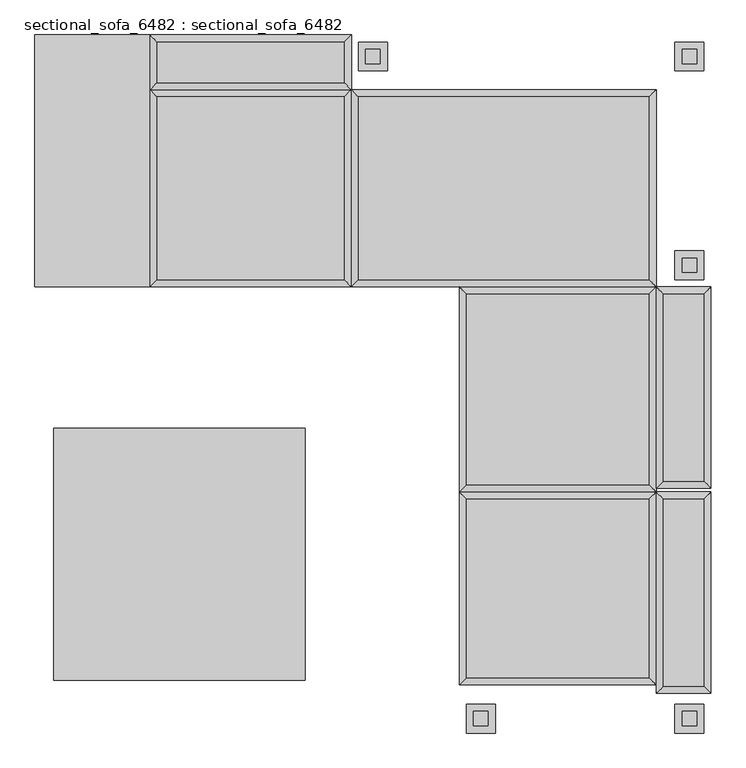
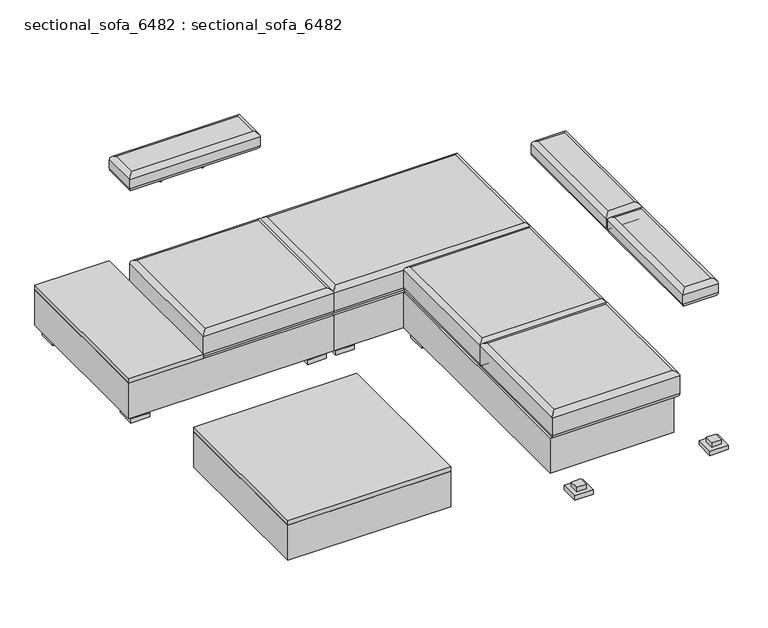
"""IFC4 building model written with IfcOpenShell, lengths in millimetres: proxy geometry, sectional_sofa_6482 : sectional_sofa_6482."""

from ifc_helpers import new_model, si_unit, point, frame, frame_2d, origin, place, context, project, spatial, polyline, circle_curve, ellipse_curve, trimmed, segment, composite_curve, outline, extrude, faceted_brep, source, transform, mapped, element, save
from ifc_brep_helpers import plane_surface, cylinder_surface, advanced_brep


def sectional_sofa_6482_sectional_sofa_6482_559db2f0(model_context):
    return source(origin(), model_context, "Body", "SolidModel", [
        extrude(outline(polyline([(-712.932438, 1291.6931081), (-712.932438, 1077.8583572), (-1.732438, 1077.8583572), (-1.732438, 402.6931081), (-1119.332438, 402.6931081), (-1119.332438, 1291.6931081), (-712.932438, 1291.6931081)])), frame((0.0, 0.0, 50.8), z_axis=(0.0, 0.0, 1.0), x_axis=(1.0, 0.0, 0.0)), (0.0, 0.0, 1.0), 203.2),
        extrude(outline(polyline([(1054.4328112, 1077.8583572), (1054.4328112, 402.6931081), (-1.732438, 402.6931081), (-1.732438, 1077.8583572), (1054.4328112, 1077.8583572)])), frame((0.0, 0.0, 50.8), z_axis=(0.0, 0.0, 1.0), x_axis=(1.0, 0.0, 0.0)), (0.0, 0.0, 1.0), 203.2),
        extrude(outline(polyline([(1054.4328112, -983.672141), (379.267562, -983.672141), (379.267562, 402.6931081), (1054.4328112, 402.6931081), (1054.4328112, -983.672141)])), frame((0.0, 0.0, 50.8), z_axis=(0.0, 0.0, 1.0), x_axis=(1.0, 0.0, 0.0)), (0.0, 0.0, 1.0), 203.2),
        faceted_brep([(-712.932438, 1291.6931081, 279.4), (-1119.332438, 1291.6931081, 279.4), (-1119.332438, 402.6931081, 279.4), (-712.932438, 402.6931081, 279.4), (-712.932438, 1098.2849958, 279.4), (-712.932438, 402.6931081, 254.0), (-1119.332438, 402.6931081, 254.0), (-1119.332438, 1291.6931081, 254.0), (-712.932438, 1291.6931081, 254.0), (-712.932438, 1098.2849958, 254.0)], [[[0, 1, 2, 3, 4]], [[5, 6, 7, 8, 9]], [[1, 0, 8, 7]], [[2, 1, 7, 6]], [[3, 2, 6, 5]], [[8, 0, 4, 3, 5, 9]]]),
        advanced_brep(
        [(404.667562, -346.6068919, 406.4), (404.667562, -977.0009907, 406.4), (1049.4594497, -977.0009907, 406.4), (1049.4594497, -346.6068919, 406.4), (404.667562, -977.0009907, 254.0), (404.667562, -346.6068919, 254.0), (1049.4594497, -346.6068919, 254.0), (1049.4594497, -977.0009907, 254.0), (1074.8594497, -321.2068919, 279.4), (1074.8594497, -321.2068919, 381.0), (1074.8594497, -1002.4009907, 381.0), (1074.8594497, -1002.4009907, 279.4), (379.267562, -321.2068919, 279.4), (379.267562, -321.2068919, 381.0), (379.267562, -1002.4009907, 279.4), (379.267562, -1002.4009907, 381.0)],
        [
            (0, 1),
            (1, 2),
            (2, 3),
            (3, 0),
            (4, 5),
            (5, 6),
            (6, 7),
            (7, 4),
            (8, 9),
            (9, 10),
            (10, 11),
            (11, 8),
            (8, 12),
            (12, 13),
            (13, 9),
            (12, 14),
            (14, 15),
            (15, 13),
            (10, 15),
            (14, 11),
            (15, 1, ellipse_curve(frame((404.667562, -977.0009907, 381.0), z_axis=(-0.7071067811865459, 0.707106781186549, 0.0), x_axis=(-0.7071067811865489, -0.7071067811865462, 0.0)), 35.9210245, 25.4)),
            (0, 13, ellipse_curve(frame((404.667562, -346.6068919, 381.0), z_axis=(-0.7071067811865489, -0.707106781186546, 0.0), x_axis=(0.707106781186546, -0.7071067811865489, 0.0)), 35.9210245, 25.4)),
            (4, 14, ellipse_curve(frame((404.667562, -977.0009907, 279.4), z_axis=(-0.7071067811865459, 0.707106781186549, 0.0), x_axis=(-0.7071067811865489, -0.7071067811865462, 0.0)), 35.9210245, 25.4)),
            (12, 5, ellipse_curve(frame((404.667562, -346.6068919, 279.4), z_axis=(-0.7071067811865489, -0.707106781186546, 0.0), x_axis=(0.707106781186546, -0.7071067811865489, 0.0)), 35.9210245, 25.4)),
            (10, 2, ellipse_curve(frame((1049.4594497, -977.0009907, 381.0), z_axis=(-0.707106781186549, -0.707106781186546, 0.0), x_axis=(0.7071067811865461, -0.7071067811865489, 0.0)), 35.9210245, 25.4)),
            (7, 11, ellipse_curve(frame((1049.4594497, -977.0009907, 279.4), z_axis=(-0.707106781186549, -0.707106781186546, 0.0), x_axis=(0.7071067811865461, -0.7071067811865489, 0.0)), 35.9210245, 25.4)),
            (9, 3, ellipse_curve(frame((1049.4594497, -346.6068919, 381.0), z_axis=(0.7071067811865461, -0.7071067811865489, 0.0), x_axis=(0.7071067811865489, 0.7071067811865461, 0.0)), 35.9210245, 25.4)),
            (6, 8, ellipse_curve(frame((1049.4594497, -346.6068919, 279.4), z_axis=(0.7071067811865461, -0.7071067811865489, 0.0), x_axis=(0.7071067811865489, 0.7071067811865461, 0.0)), 35.9210245, 25.4)),
        ],
        [
            plane_surface(frame((1074.8594497, -333.9068919, 406.4), z_axis=(0.0, 0.0, 1.0), x_axis=(0.0, 1.0, 0.0))),
            plane_surface(frame((1074.8594497, -333.9068919, 254.0), z_axis=(0.0, 0.0, -1.0), x_axis=(0.0, -1.0, 0.0))),
            plane_surface(frame((1074.8594497, -1002.4009907, 406.4), z_axis=(1.0, 0.0, 0.0), x_axis=(0.0, 0.0, -1.0))),
            plane_surface(frame((1074.8594497, -321.2068919, 406.4), z_axis=(0.0, 1.0, 0.0), x_axis=(0.0, 0.0, -1.0))),
            plane_surface(frame((379.267562, -321.2068919, 406.4), z_axis=(-1.0, 0.0, 0.0), x_axis=(0.0, 0.0, -1.0))),
            plane_surface(frame((379.267562, -1002.4009907, 406.4), z_axis=(0.0, -1.0, 0.0), x_axis=(0.0, 0.0, -1.0))),
            cylinder_surface(frame((404.667562, -321.2068919, 381.0), z_axis=(0.0, -1.0, 0.0), x_axis=(1.0, 0.0, 0.0)), 25.4),
            cylinder_surface(frame((404.667562, -321.2068919, 279.4), z_axis=(0.0, -1.0, 0.0), x_axis=(1.0, 0.0, 0.0)), 25.4),
            cylinder_surface(frame((379.267562, -977.0009907, 381.0), z_axis=(1.0, 0.0, 0.0), x_axis=(0.0, 1.0, 0.0)), 25.4),
            cylinder_surface(frame((379.267562, -977.0009907, 279.4), z_axis=(1.0, 0.0, 0.0), x_axis=(0.0, 1.0, 0.0)), 25.4),
            cylinder_surface(frame((1049.4594497, -1002.4009907, 381.0), z_axis=(0.0, 1.0, 0.0), x_axis=(-1.0, 0.0, 0.0)), 25.4),
            cylinder_surface(frame((1049.4594497, -1002.4009907, 279.4), z_axis=(0.0, 1.0, 0.0), x_axis=(-1.0, 0.0, 0.0)), 25.4),
            cylinder_surface(frame((1074.8594497, -346.6068919, 381.0), z_axis=(-1.0, 0.0, 0.0), x_axis=(0.0, -1.0, 0.0)), 25.4),
            cylinder_surface(frame((1074.8594497, -346.6068919, 279.4), z_axis=(-1.0, 0.0, 0.0), x_axis=(0.0, -1.0, 0.0)), 25.4),
        ],
        [
            (0, [[1, 2, 3, 4]]),
            (1, [[5, 6, 7, 8]]),
            (2, [[9, 10, 11, 12]]),
            (3, [[-9, 13, 14, 15]]),
            (4, [[-14, 16, 17, 18]]),
            (5, [[-11, 19, -17, 20]]),
            (6, [[21, -1, 22, -18]]),
            (7, [[23, -16, 24, -5]]),
            (8, [[-21, -19, 25, -2]]),
            (9, [[-23, -8, 26, -20]]),
            (10, [[-25, -10, 27, -3]]),
            (11, [[-26, -7, 28, -12]]),
            (12, [[-22, -4, -27, -15]]),
            (13, [[-24, -13, -28, -6]]),
        ],
    ),
        faceted_brep([(-992.332438, 1164.6931081, 25.4), (-992.332438, 1266.2931081, 25.4), (-1093.932438, 1266.2931081, 25.4), (-1093.932438, 1164.6931081, 25.4), (-1017.732438, 1240.8931081, 25.4), (-1017.732438, 1190.0931081, 25.4), (-1068.532438, 1190.0931081, 25.4), (-1068.532438, 1240.8931081, 25.4), (-992.332438, 1164.6931081, 0.0), (-1093.932438, 1164.6931081, 0.0), (-1093.932438, 1266.2931081, 0.0), (-992.332438, 1266.2931081, 0.0), (-1017.732438, 1190.0931081, 50.8), (-1017.732438, 1240.8931081, 50.8), (-1068.532438, 1240.8931081, 50.8), (-1068.532438, 1190.0931081, 50.8)], [[[0, 1, 2, 3], [4, 5, 6, 7]], [[8, 9, 10, 11]], [[1, 0, 8, 11]], [[2, 1, 11, 10]], [[3, 2, 10, 9]], [[0, 3, 9, 8]], [[12, 13, 14, 15]], [[13, 12, 5, 4]], [[14, 13, 4, 7]], [[15, 14, 7, 6]], [[12, 15, 6, 5]]]),
        faceted_brep([(-992.332438, 428.0931081, 25.4), (-992.332438, 529.6931081, 25.4), (-1093.932438, 529.6931081, 25.4), (-1093.932438, 428.0931081, 25.4), (-1017.732438, 504.2931081, 25.4), (-1017.732438, 453.4931081, 25.4), (-1068.532438, 453.4931081, 25.4), (-1068.532438, 504.2931081, 25.4), (-992.332438, 428.0931081, 0.0), (-1093.932438, 428.0931081, 0.0), (-1093.932438, 529.6931081, 0.0), (-992.332438, 529.6931081, 0.0), (-1017.732438, 453.4931081, 50.8), (-1017.732438, 504.2931081, 50.8), (-1068.532438, 504.2931081, 50.8), (-1068.532438, 453.4931081, 50.8)], [[[0, 1, 2, 3], [4, 5, 6, 7]], [[8, 9, 10, 11]], [[1, 0, 8, 11]], [[2, 1, 11, 10]], [[3, 2, 10, 9]], [[0, 3, 9, 8]], [[12, 13, 14, 15]], [[13, 12, 5, 4]], [[14, 13, 4, 7]], [[15, 14, 7, 6]], [[12, 15, 6, 5]]]),
        faceted_brep([(-27.132438, 1164.6931081, 25.4), (-27.132438, 1266.2931081, 25.4), (-128.732438, 1266.2931081, 25.4), (-128.732438, 1164.6931081, 25.4), (-52.532438, 1240.8931081, 25.4), (-52.532438, 1190.0931081, 25.4), (-103.332438, 1190.0931081, 25.4), (-103.332438, 1240.8931081, 25.4), (-27.132438, 1164.6931081, 0.0), (-128.732438, 1164.6931081, 0.0), (-128.732438, 1266.2931081, 0.0), (-27.132438, 1266.2931081, 0.0), (-52.532438, 1190.0931081, 50.8), (-52.532438, 1240.8931081, 50.8), (-103.332438, 1240.8931081, 50.8), (-103.332438, 1190.0931081, 50.8)], [[[0, 1, 2, 3], [4, 5, 6, 7]], [[8, 9, 10, 11]], [[1, 0, 8, 11]], [[2, 1, 11, 10]], [[3, 2, 10, 9]], [[0, 3, 9, 8]], [[12, 13, 14, 15]], [[13, 12, 5, 4]], [[14, 13, 4, 7]], [[15, 14, 7, 6]], [[12, 15, 6, 5]]]),
        faceted_brep([(23.667562, 1164.6931081, 25.4), (125.267562, 1164.6931081, 25.4), (125.267562, 1266.2931081, 25.4), (23.667562, 1266.2931081, 25.4), (99.867562, 1190.0931081, 25.4), (49.067562, 1190.0931081, 25.4), (49.067562, 1240.8931081, 25.4), (99.867562, 1240.8931081, 25.4), (23.667562, 1164.6931081, 0.0), (23.667562, 1266.2931081, 0.0), (125.267562, 1266.2931081, 0.0), (125.267562, 1164.6931081, 0.0), (49.067562, 1190.0931081, 50.8), (99.867562, 1190.0931081, 50.8), (99.867562, 1240.8931081, 50.8), (49.067562, 1240.8931081, 50.8)], [[[0, 1, 2, 3], [4, 5, 6, 7]], [[8, 9, 10, 11]], [[1, 0, 8, 11]], [[2, 1, 11, 10]], [[3, 2, 10, 9]], [[0, 3, 9, 8]], [[12, 13, 14, 15]], [[13, 12, 5, 4]], [[14, 13, 4, 7]], [[15, 14, 7, 6]], [[12, 15, 6, 5]]]),
        faceted_brep([(-27.132438, 428.0931081, 25.4), (-27.132438, 529.6931081, 25.4), (-128.732438, 529.6931081, 25.4), (-128.732438, 428.0931081, 25.4), (-52.532438, 504.2931081, 25.4), (-52.532438, 453.4931081, 25.4), (-103.332438, 453.4931081, 25.4), (-103.332438, 504.2931081, 25.4), (-27.132438, 428.0931081, 0.0), (-128.732438, 428.0931081, 0.0), (-128.732438, 529.6931081, 0.0), (-27.132438, 529.6931081, 0.0), (-52.532438, 453.4931081, 50.8), (-52.532438, 504.2931081, 50.8), (-103.332438, 504.2931081, 50.8), (-103.332438, 453.4931081, 50.8)], [[[0, 1, 2, 3], [4, 5, 6, 7]], [[8, 9, 10, 11]], [[1, 0, 8, 11]], [[2, 1, 11, 10]], [[3, 2, 10, 9]], [[0, 3, 9, 8]], [[12, 13, 14, 15]], [[13, 12, 5, 4]], [[14, 13, 4, 7]], [[15, 14, 7, 6]], [[12, 15, 6, 5]]]),
        faceted_brep([(23.667562, 428.0931081, 25.4), (125.267562, 428.0931081, 25.4), (125.267562, 529.6931081, 25.4), (23.667562, 529.6931081, 25.4), (99.867562, 453.4931081, 25.4), (49.067562, 453.4931081, 25.4), (49.067562, 504.2931081, 25.4), (99.867562, 504.2931081, 25.4), (23.667562, 428.0931081, 0.0), (23.667562, 529.6931081, 0.0), (125.267562, 529.6931081, 0.0), (125.267562, 428.0931081, 0.0), (49.067562, 453.4931081, 50.8), (99.867562, 453.4931081, 50.8), (99.867562, 504.2931081, 50.8), (49.067562, 504.2931081, 50.8)], [[[0, 1, 2, 3], [4, 5, 6, 7]], [[8, 9, 10, 11]], [[1, 0, 8, 11]], [[2, 1, 11, 10]], [[3, 2, 10, 9]], [[0, 3, 9, 8]], [[12, 13, 14, 15]], [[13, 12, 5, 4]], [[14, 13, 4, 7]], [[15, 14, 7, 6]], [[12, 15, 6, 5]]]),
        faceted_brep([(1242.867562, 1164.6931081, 25.4), (1242.867562, 1266.2931081, 25.4), (1141.267562, 1266.2931081, 25.4), (1141.267562, 1164.6931081, 25.4), (1217.467562, 1240.8931081, 25.4), (1217.467562, 1190.0931081, 25.4), (1166.667562, 1190.0931081, 25.4), (1166.667562, 1240.8931081, 25.4), (1242.867562, 1164.6931081, 0.0), (1141.267562, 1164.6931081, 0.0), (1141.267562, 1266.2931081, 0.0), (1242.867562, 1266.2931081, 0.0), (1217.467562, 1190.0931081, 50.8), (1217.467562, 1240.8931081, 50.8), (1166.667562, 1240.8931081, 50.8), (1166.667562, 1190.0931081, 50.8)], [[[0, 1, 2, 3], [4, 5, 6, 7]], [[8, 9, 10, 11]], [[1, 0, 8, 11]], [[2, 1, 11, 10]], [[3, 2, 10, 9]], [[0, 3, 9, 8]], [[12, 13, 14, 15]], [[13, 12, 5, 4]], [[14, 13, 4, 7]], [[15, 14, 7, 6]], [[12, 15, 6, 5]]]),
        faceted_brep([(506.267562, 377.2931081, 25.4), (404.667562, 377.2931081, 25.4), (404.667562, 275.6931081, 25.4), (506.267562, 275.6931081, 25.4), (430.067562, 351.8931081, 25.4), (480.867562, 351.8931081, 25.4), (480.867562, 301.0931081, 25.4), (430.067562, 301.0931081, 25.4), (506.267562, 377.2931081, 0.0), (506.267562, 275.6931081, 0.0), (404.667562, 275.6931081, 0.0), (404.667562, 377.2931081, 0.0), (480.867562, 351.8931081, 50.8), (430.067562, 351.8931081, 50.8), (430.067562, 301.0931081, 50.8), (480.867562, 301.0931081, 50.8)], [[[0, 1, 2, 3], [4, 5, 6, 7]], [[8, 9, 10, 11]], [[1, 0, 8, 11]], [[2, 1, 11, 10]], [[3, 2, 10, 9]], [[0, 3, 9, 8]], [[12, 13, 14, 15]], [[13, 12, 5, 4]], [[14, 13, 4, 7]], [[15, 14, 7, 6]], [[12, 15, 6, 5]]]),
        faceted_brep([(1242.867562, 428.0931081, 25.4), (1242.867562, 529.6931081, 25.4), (1141.267562, 529.6931081, 25.4), (1141.267562, 428.0931081, 25.4), (1217.467562, 504.2931081, 25.4), (1217.467562, 453.4931081, 25.4), (1166.667562, 453.4931081, 25.4), (1166.667562, 504.2931081, 25.4), (1242.867562, 428.0931081, 0.0), (1141.267562, 428.0931081, 0.0), (1141.267562, 529.6931081, 0.0), (1242.867562, 529.6931081, 0.0), (1217.467562, 453.4931081, 50.8), (1217.467562, 504.2931081, 50.8), (1166.667562, 504.2931081, 50.8), (1166.667562, 453.4931081, 50.8)], [[[0, 1, 2, 3], [4, 5, 6, 7]], [[8, 9, 10, 11]], [[1, 0, 8, 11]], [[2, 1, 11, 10]], [[3, 2, 10, 9]], [[0, 3, 9, 8]], [[12, 13, 14, 15]], [[13, 12, 5, 4]], [[14, 13, 4, 7]], [[15, 14, 7, 6]], [[12, 15, 6, 5]]]),
        faceted_brep([(1242.867562, 377.2931081, 25.4), (1141.267562, 377.2931081, 25.4), (1141.267562, 275.6931081, 25.4), (1242.867562, 275.6931081, 25.4), (1166.667562, 351.8931081, 25.4), (1217.467562, 351.8931081, 25.4), (1217.467562, 301.0931081, 25.4), (1166.667562, 301.0931081, 25.4), (1242.867562, 377.2931081, 0.0), (1242.867562, 275.6931081, 0.0), (1141.267562, 275.6931081, 0.0), (1141.267562, 377.2931081, 0.0), (1217.467562, 351.8931081, 50.8), (1166.667562, 351.8931081, 50.8), (1166.667562, 301.0931081, 50.8), (1217.467562, 301.0931081, 50.8)], [[[0, 1, 2, 3], [4, 5, 6, 7]], [[8, 9, 10, 11]], [[1, 0, 8, 11]], [[2, 1, 11, 10]], [[3, 2, 10, 9]], [[0, 3, 9, 8]], [[12, 13, 14, 15]], [[13, 12, 5, 4]], [[14, 13, 4, 7]], [[15, 14, 7, 6]], [[12, 15, 6, 5]]]),
        faceted_brep([(506.267562, -1172.1068919, 25.4), (506.267562, -1070.5068919, 25.4), (404.667562, -1070.5068919, 25.4), (404.667562, -1172.1068919, 25.4), (480.867562, -1095.9068919, 25.4), (480.867562, -1146.7068919, 25.4), (430.067562, -1146.7068919, 25.4), (430.067562, -1095.9068919, 25.4), (506.267562, -1172.1068919, 0.0), (404.667562, -1172.1068919, 0.0), (404.667562, -1070.5068919, 0.0), (506.267562, -1070.5068919, 0.0), (480.867562, -1146.7068919, 50.8), (480.867562, -1095.9068919, 50.8), (430.067562, -1095.9068919, 50.8), (430.067562, -1146.7068919, 50.8)], [[[0, 1, 2, 3], [4, 5, 6, 7]], [[8, 9, 10, 11]], [[1, 0, 8, 11]], [[2, 1, 11, 10]], [[3, 2, 10, 9]], [[0, 3, 9, 8]], [[12, 13, 14, 15]], [[13, 12, 5, 4]], [[14, 13, 4, 7]], [[15, 14, 7, 6]], [[12, 15, 6, 5]]]),
        faceted_brep([(1242.867562, -1172.1068919, 25.4), (1242.867562, -1070.5068919, 25.4), (1141.267562, -1070.5068919, 25.4), (1141.267562, -1172.1068919, 25.4), (1217.467562, -1095.9068919, 25.4), (1217.467562, -1146.7068919, 25.4), (1166.667562, -1146.7068919, 25.4), (1166.667562, -1095.9068919, 25.4), (1242.867562, -1172.1068919, 0.0), (1141.267562, -1172.1068919, 0.0), (1141.267562, -1070.5068919, 0.0), (1242.867562, -1070.5068919, 0.0), (1217.467562, -1146.7068919, 50.8), (1217.467562, -1095.9068919, 50.8), (1166.667562, -1095.9068919, 50.8), (1166.667562, -1146.7068919, 50.8)], [[[0, 1, 2, 3], [4, 5, 6, 7]], [[8, 9, 10, 11]], [[1, 0, 8, 11]], [[2, 1, 11, 10]], [[3, 2, 10, 9]], [[0, 3, 9, 8]], [[12, 13, 14, 15]], [[13, 12, 5, 4]], [[14, 13, 4, 7]], [[15, 14, 7, 6]], [[12, 15, 6, 5]]]),
        extrude(outline(composite_curve([segment(trimmed(circle_curve(frame_2d((-482.8859111, 1206.7842798)), 6.35), [point((-489.2359111, 1206.7842798))], [point((-476.5359111, 1206.7842798))], False, "CARTESIAN"), True, "CONTINUOUS"), segment(trimmed(circle_curve(frame_2d((-482.8859111, 1206.7842798)), 6.35), [point((-476.5359111, 1206.7842798))], [point((-489.2359111, 1206.7842798))], False, "CARTESIAN"), True, "CONTINUOUS")], self_intersect=False)), frame((0.0, 0.0, 711.2), z_axis=(0.0, 0.0, 1.0), x_axis=(1.0, 0.0, 0.0)), (0.0, 0.0, 1.0), 76.2),
        extrude(outline(composite_curve([segment(trimmed(circle_curve(frame_2d((-254.2859111, 1206.7842798)), 6.35), [point((-260.6359111, 1206.7842798))], [point((-247.9359111, 1206.7842798))], False, "CARTESIAN"), True, "CONTINUOUS"), segment(trimmed(circle_curve(frame_2d((-254.2859111, 1206.7842798)), 6.35), [point((-247.9359111, 1206.7842798))], [point((-260.6359111, 1206.7842798))], False, "CARTESIAN"), True, "CONTINUOUS")], self_intersect=False)), frame((0.0, 0.0, 711.2), z_axis=(0.0, 0.0, 1.0), x_axis=(1.0, 0.0, 0.0)), (0.0, 0.0, 1.0), 76.2),
        extrude(outline(composite_curve([segment(trimmed(circle_curve(frame_2d((1173.6454882, 148.0415505)), 6.35), [point((1173.6454882, 154.3915505))], [point((1173.6454882, 141.6915505))], False, "CARTESIAN"), True, "CONTINUOUS"), segment(trimmed(circle_curve(frame_2d((1173.6454882, 148.0415505)), 6.35), [point((1173.6454882, 141.6915505))], [point((1173.6454882, 154.3915505))], False, "CARTESIAN"), True, "CONTINUOUS")], self_intersect=False)), frame((0.0, 0.0, 711.2), z_axis=(0.0, 0.0, 1.0), x_axis=(1.0, 0.0, 0.0)), (0.0, 0.0, 1.0), 76.2),
        extrude(outline(composite_curve([segment(trimmed(circle_curve(frame_2d((1173.6454882, -80.5584495)), 6.35), [point((1173.6454882, -74.2084495))], [point((1173.6454882, -86.9084495))], False, "CARTESIAN"), True, "CONTINUOUS"), segment(trimmed(circle_curve(frame_2d((1173.6454882, -80.5584495)), 6.35), [point((1173.6454882, -86.9084495))], [point((1173.6454882, -74.2084495))], False, "CARTESIAN"), True, "CONTINUOUS")], self_intersect=False)), frame((0.0, 0.0, 711.2), z_axis=(0.0, 0.0, 1.0), x_axis=(1.0, 0.0, 0.0)), (0.0, 0.0, 1.0), 76.2),
        extrude(outline(composite_curve([segment(trimmed(circle_curve(frame_2d((1173.6454882, -563.1584495)), 6.35), [point((1173.6454882, -556.8084495))], [point((1173.6454882, -569.5084495))], False, "CARTESIAN"), True, "CONTINUOUS"), segment(trimmed(circle_curve(frame_2d((1173.6454882, -563.1584495)), 6.35), [point((1173.6454882, -569.5084495))], [point((1173.6454882, -556.8084495))], False, "CARTESIAN"), True, "CONTINUOUS")], self_intersect=False)), frame((0.0, 0.0, 711.2), z_axis=(0.0, 0.0, 1.0), x_axis=(1.0, 0.0, 0.0)), (0.0, 0.0, 1.0), 76.2),
        extrude(outline(composite_curve([segment(trimmed(circle_curve(frame_2d((1173.6454882, -791.7584495)), 6.35), [point((1173.6454882, -785.4084495))], [point((1173.6454882, -798.1084495))], False, "CARTESIAN"), True, "CONTINUOUS"), segment(trimmed(circle_curve(frame_2d((1173.6454882, -791.7584495)), 6.35), [point((1173.6454882, -798.1084495))], [point((1173.6454882, -785.4084495))], False, "CARTESIAN"), True, "CONTINUOUS")], self_intersect=False)), frame((0.0, 0.0, 711.2), z_axis=(0.0, 0.0, 1.0), x_axis=(1.0, 0.0, 0.0)), (0.0, 0.0, 1.0), 76.2),
        advanced_brep(
        [(-687.532438, 1123.6849958, 889.0), (-27.132438, 1123.6849958, 889.0), (-27.132438, 1266.2931081, 889.0), (-687.532438, 1266.2931081, 889.0), (-27.132438, 1123.6849958, 787.4), (-687.532438, 1123.6849958, 787.4), (-687.532438, 1266.2931081, 787.4), (-27.132438, 1266.2931081, 787.4), (-1.732438, 1291.6931081, 863.6), (-1.732438, 1291.6931081, 812.8), (-712.932438, 1291.6931081, 812.8), (-712.932438, 1291.6931081, 863.6), (-712.932438, 1098.2849958, 812.8), (-712.932438, 1098.2849958, 863.6), (-1.732438, 1098.2849958, 812.8), (-1.732438, 1098.2849958, 863.6)],
        [
            (0, 1),
            (1, 2),
            (2, 3),
            (3, 0),
            (4, 5),
            (5, 6),
            (6, 7),
            (7, 4),
            (8, 9),
            (9, 10),
            (10, 11),
            (11, 8),
            (10, 12),
            (12, 13),
            (13, 11),
            (12, 14),
            (14, 15),
            (15, 13),
            (8, 15),
            (14, 9),
            (15, 1, ellipse_curve(frame((-27.132438, 1123.6849958, 863.6), z_axis=(-0.7071067811865475, -0.7071067811865475, 0.0), x_axis=(0.7071067811865476, -0.7071067811865474, 0.0)), 35.9210245, 25.4)),
            (0, 13, ellipse_curve(frame((-687.532438, 1123.6849958, 863.6), z_axis=(0.7071067811865475, -0.7071067811865475, 0.0), x_axis=(0.7071067811865476, 0.7071067811865474, 0.0)), 35.9210245, 25.4)),
            (4, 14, ellipse_curve(frame((-27.132438, 1123.6849958, 812.8), z_axis=(-0.7071067811865475, -0.7071067811865475, 0.0), x_axis=(0.7071067811865476, -0.7071067811865474, 0.0)), 35.9210245, 25.4)),
            (12, 5, ellipse_curve(frame((-687.532438, 1123.6849958, 812.8), z_axis=(0.7071067811865475, -0.7071067811865475, 0.0), x_axis=(0.7071067811865476, 0.7071067811865474, 0.0)), 35.9210245, 25.4)),
            (8, 2, ellipse_curve(frame((-27.132438, 1266.2931081, 863.6), z_axis=(0.7071067811865475, -0.7071067811865475, 0.0), x_axis=(0.7071067811865474, 0.7071067811865476, 0.0)), 35.9210245, 25.4)),
            (7, 9, ellipse_curve(frame((-27.132438, 1266.2931081, 812.8), z_axis=(0.7071067811865475, -0.7071067811865475, 0.0), x_axis=(0.7071067811865474, 0.7071067811865476, 0.0)), 35.9210245, 25.4)),
            (11, 3, ellipse_curve(frame((-687.532438, 1266.2931081, 863.6), z_axis=(0.7071067811865475, 0.7071067811865475, 0.0), x_axis=(-0.7071067811865476, 0.7071067811865474, 0.0)), 35.9210245, 25.4)),
            (6, 10, ellipse_curve(frame((-687.532438, 1266.2931081, 812.8), z_axis=(0.7071067811865475, 0.7071067811865475, 0.0), x_axis=(-0.7071067811865476, 0.7071067811865474, 0.0)), 35.9210245, 25.4)),
        ],
        [
            plane_surface(frame((-712.932438, 1291.6931081, 889.0), z_axis=(0.0, 0.0, 1.0), x_axis=(-1.0, 0.0, 0.0))),
            plane_surface(frame((-712.932438, 1291.6931081, 787.4), z_axis=(0.0, 0.0, -1.0), x_axis=(1.0, 0.0, 0.0))),
            plane_surface(frame((-1.732438, 1291.6931081, 889.0), z_axis=(0.0, 1.0, 0.0), x_axis=(0.0, 0.0, -1.0))),
            plane_surface(frame((-712.932438, 1291.6931081, 889.0), z_axis=(-1.0, 0.0, 0.0), x_axis=(0.0, 0.0, -1.0))),
            plane_surface(frame((-712.932438, 1098.2849958, 889.0), z_axis=(0.0, -1.0, 0.0), x_axis=(0.0, 0.0, -1.0))),
            plane_surface(frame((-1.732438, 1098.2849958, 889.0), z_axis=(1.0, 0.0, 0.0), x_axis=(0.0, 0.0, -1.0))),
            cylinder_surface(frame((-712.932438, 1123.6849958, 863.6), z_axis=(1.0, 0.0, 0.0), x_axis=(0.0, 1.0, 0.0)), 25.4),
            cylinder_surface(frame((-712.932438, 1123.6849958, 812.8), z_axis=(1.0, 0.0, 0.0), x_axis=(0.0, 1.0, 0.0)), 25.4),
            cylinder_surface(frame((-27.132438, 1098.2849958, 863.6), z_axis=(0.0, 1.0, 0.0), x_axis=(-1.0, 0.0, 0.0)), 25.4),
            cylinder_surface(frame((-27.132438, 1098.2849958, 812.8), z_axis=(0.0, 1.0, 0.0), x_axis=(-1.0, 0.0, 0.0)), 25.4),
            cylinder_surface(frame((-1.732438, 1266.2931081, 863.6), z_axis=(-1.0, 0.0, 0.0), x_axis=(0.0, -1.0, 0.0)), 25.4),
            cylinder_surface(frame((-1.732438, 1266.2931081, 812.8), z_axis=(-1.0, 0.0, 0.0), x_axis=(0.0, -1.0, 0.0)), 25.4),
            cylinder_surface(frame((-687.532438, 1291.6931081, 863.6), z_axis=(0.0, -1.0, 0.0), x_axis=(1.0, 0.0, 0.0)), 25.4),
            cylinder_surface(frame((-687.532438, 1291.6931081, 812.8), z_axis=(0.0, -1.0, 0.0), x_axis=(1.0, 0.0, 0.0)), 25.4),
        ],
        [
            (0, [[1, 2, 3, 4]]),
            (1, [[5, 6, 7, 8]]),
            (2, [[9, 10, 11, 12]]),
            (3, [[-11, 13, 14, 15]]),
            (4, [[-14, 16, 17, 18]]),
            (5, [[-9, 19, -17, 20]]),
            (6, [[21, -1, 22, -18]]),
            (7, [[23, -16, 24, -5]]),
            (8, [[-21, -19, 25, -2]]),
            (9, [[-23, -8, 26, -20]]),
            (10, [[-25, -12, 27, -3]]),
            (11, [[-26, -7, 28, -10]]),
            (12, [[-22, -4, -27, -15]]),
            (13, [[-24, -13, -28, -6]]),
        ],
    ),
        advanced_brep(
        [(1100.2594497, 377.2931081, 889.0), (1100.2594497, -283.1068919, 889.0), (1242.867562, -283.1068919, 889.0), (1242.867562, 377.2931081, 889.0), (1100.2594497, -283.1068919, 787.4), (1100.2594497, 377.2931081, 787.4), (1242.867562, 377.2931081, 787.4), (1242.867562, -283.1068919, 787.4), (1268.267562, -308.5068919, 863.6), (1268.267562, -308.5068919, 812.8), (1268.267562, 402.6931081, 812.8), (1268.267562, 402.6931081, 863.6), (1074.8594497, 402.6931081, 812.8), (1074.8594497, 402.6931081, 863.6), (1074.8594497, -308.5068919, 812.8), (1074.8594497, -308.5068919, 863.6)],
        [
            (0, 1),
            (1, 2),
            (2, 3),
            (3, 0),
            (4, 5),
            (5, 6),
            (6, 7),
            (7, 4),
            (8, 9),
            (9, 10),
            (10, 11),
            (11, 8),
            (10, 12),
            (12, 13),
            (13, 11),
            (12, 14),
            (14, 15),
            (15, 13),
            (8, 15),
            (14, 9),
            (15, 1, ellipse_curve(frame((1100.2594497, -283.1068919, 863.6), z_axis=(-0.7071067811865487, 0.7071067811865462, 0.0), x_axis=(-0.7071067811865462, -0.7071067811865488, 0.0)), 35.9210245, 25.4)),
            (0, 13, ellipse_curve(frame((1100.2594497, 377.2931081, 863.6), z_axis=(-0.7071067811865461, -0.7071067811865489, 0.0), x_axis=(0.7071067811865489, -0.7071067811865461, 0.0)), 35.9210245, 25.4)),
            (4, 14, ellipse_curve(frame((1100.2594497, -283.1068919, 812.8), z_axis=(-0.7071067811865487, 0.7071067811865462, 0.0), x_axis=(-0.7071067811865462, -0.7071067811865488, 0.0)), 35.9210245, 25.4)),
            (12, 5, ellipse_curve(frame((1100.2594497, 377.2931081, 812.8), z_axis=(-0.7071067811865461, -0.7071067811865489, 0.0), x_axis=(0.7071067811865489, -0.7071067811865461, 0.0)), 35.9210245, 25.4)),
            (8, 2, ellipse_curve(frame((1242.867562, -283.1068919, 863.6), z_axis=(-0.7071067811865462, -0.7071067811865489, 0.0), x_axis=(0.7071067811865487, -0.7071067811865464, 0.0)), 35.9210245, 25.4)),
            (7, 9, ellipse_curve(frame((1242.867562, -283.1068919, 812.8), z_axis=(-0.7071067811865462, -0.7071067811865489, 0.0), x_axis=(0.7071067811865487, -0.7071067811865464, 0.0)), 35.9210245, 25.4)),
            (11, 3, ellipse_curve(frame((1242.867562, 377.2931081, 863.6), z_axis=(0.707106781186549, -0.707106781186546, 0.0), x_axis=(0.707106781186546, 0.707106781186549, 0.0)), 35.9210245, 25.4)),
            (6, 10, ellipse_curve(frame((1242.867562, 377.2931081, 812.8), z_axis=(0.707106781186549, -0.707106781186546, 0.0), x_axis=(0.707106781186546, 0.707106781186549, 0.0)), 35.9210245, 25.4)),
        ],
        [
            plane_surface(frame((1268.267562, 402.6931081, 889.0), z_axis=(0.0, 0.0, 1.0), x_axis=(0.0, 1.0, 0.0))),
            plane_surface(frame((1268.267562, 402.6931081, 787.4), z_axis=(0.0, 0.0, -1.0), x_axis=(0.0, -1.0, 0.0))),
            plane_surface(frame((1268.267562, -308.5068919, 889.0), z_axis=(1.0, 0.0, 0.0), x_axis=(0.0, 0.0, -1.0))),
            plane_surface(frame((1268.267562, 402.6931081, 889.0), z_axis=(0.0, 1.0, 0.0), x_axis=(0.0, 0.0, -1.0))),
            plane_surface(frame((1074.8594497, 402.6931081, 889.0), z_axis=(-1.0, 0.0, 0.0), x_axis=(0.0, 0.0, -1.0))),
            plane_surface(frame((1074.8594497, -308.5068919, 889.0), z_axis=(0.0, -1.0, 0.0), x_axis=(0.0, 0.0, -1.0))),
            cylinder_surface(frame((1100.2594497, 402.6931081, 863.6), z_axis=(0.0, -1.0, 0.0), x_axis=(1.0, 0.0, 0.0)), 25.4),
            cylinder_surface(frame((1100.2594497, 402.6931081, 812.8), z_axis=(0.0, -1.0, 0.0), x_axis=(1.0, 0.0, 0.0)), 25.4),
            cylinder_surface(frame((1074.8594497, -283.1068919, 863.6), z_axis=(1.0, 0.0, 0.0), x_axis=(0.0, 1.0, 0.0)), 25.4),
            cylinder_surface(frame((1074.8594497, -283.1068919, 812.8), z_axis=(1.0, 0.0, 0.0), x_axis=(0.0, 1.0, 0.0)), 25.4),
            cylinder_surface(frame((1242.867562, -308.5068919, 863.6), z_axis=(0.0, 1.0, 0.0), x_axis=(-1.0, 0.0, 0.0)), 25.4),
            cylinder_surface(frame((1242.867562, -308.5068919, 812.8), z_axis=(0.0, 1.0, 0.0), x_axis=(-1.0, 0.0, 0.0)), 25.4),
            cylinder_surface(frame((1268.267562, 377.2931081, 863.6), z_axis=(-1.0, 0.0, 0.0), x_axis=(0.0, -1.0, 0.0)), 25.4),
            cylinder_surface(frame((1268.267562, 377.2931081, 812.8), z_axis=(-1.0, 0.0, 0.0), x_axis=(0.0, -1.0, 0.0)), 25.4),
        ],
        [
            (0, [[1, 2, 3, 4]]),
            (1, [[5, 6, 7, 8]]),
            (2, [[9, 10, 11, 12]]),
            (3, [[-11, 13, 14, 15]]),
            (4, [[-14, 16, 17, 18]]),
            (5, [[-9, 19, -17, 20]]),
            (6, [[21, -1, 22, -18]]),
            (7, [[23, -16, 24, -5]]),
            (8, [[-21, -19, 25, -2]]),
            (9, [[-23, -8, 26, -20]]),
            (10, [[-25, -12, 27, -3]]),
            (11, [[-26, -7, 28, -10]]),
            (12, [[-22, -4, -27, -15]]),
            (13, [[-24, -13, -28, -6]]),
        ],
    ),
        advanced_brep(
        [(1100.2594497, -346.6068919, 889.0), (1100.2594497, -1007.0068919, 889.0), (1242.867562, -1007.0068919, 889.0), (1242.867562, -346.6068919, 889.0), (1100.2594497, -1007.0068919, 787.4), (1100.2594497, -346.6068919, 787.4), (1242.867562, -346.6068919, 787.4), (1242.867562, -1007.0068919, 787.4), (1268.267562, -1032.4068919, 863.6), (1268.267562, -1032.4068919, 812.8), (1268.267562, -321.2068919, 812.8), (1268.267562, -321.2068919, 863.6), (1074.8594497, -321.2068919, 812.8), (1074.8594497, -321.2068919, 863.6), (1074.8594497, -1032.4068919, 812.8), (1074.8594497, -1032.4068919, 863.6)],
        [
            (0, 1),
            (1, 2),
            (2, 3),
            (3, 0),
            (4, 5),
            (5, 6),
            (6, 7),
            (7, 4),
            (8, 9),
            (9, 10),
            (10, 11),
            (11, 8),
            (10, 12),
            (12, 13),
            (13, 11),
            (12, 14),
            (14, 15),
            (15, 13),
            (8, 15),
            (14, 9),
            (15, 1, ellipse_curve(frame((1100.2594497, -1007.0068919, 863.6), z_axis=(-0.7071067811865491, 0.7071067811865459, 0.0), x_axis=(-0.7071067811865458, -0.7071067811865491, 0.0)), 35.9210245, 25.4)),
            (0, 13, ellipse_curve(frame((1100.2594497, -346.6068919, 863.6), z_axis=(-0.7071067811865461, -0.7071067811865489, 0.0), x_axis=(0.7071067811865489, -0.707106781186546, 0.0)), 35.9210245, 25.4)),
            (4, 14, ellipse_curve(frame((1100.2594497, -1007.0068919, 812.8), z_axis=(-0.7071067811865491, 0.7071067811865459, 0.0), x_axis=(-0.7071067811865458, -0.7071067811865491, 0.0)), 35.9210245, 25.4)),
            (12, 5, ellipse_curve(frame((1100.2594497, -346.6068919, 812.8), z_axis=(-0.7071067811865461, -0.7071067811865489, 0.0), x_axis=(0.7071067811865489, -0.707106781186546, 0.0)), 35.9210245, 25.4)),
            (8, 2, ellipse_curve(frame((1242.867562, -1007.0068919, 863.6), z_axis=(-0.7071067811865459, -0.7071067811865491, 0.0), x_axis=(0.7071067811865491, -0.7071067811865458, 0.0)), 35.9210245, 25.4)),
            (7, 9, ellipse_curve(frame((1242.867562, -1007.0068919, 812.8), z_axis=(-0.7071067811865459, -0.7071067811865491, 0.0), x_axis=(0.7071067811865491, -0.7071067811865458, 0.0)), 35.9210245, 25.4)),
            (11, 3, ellipse_curve(frame((1242.867562, -346.6068919, 863.6), z_axis=(0.7071067811865489, -0.707106781186546, 0.0), x_axis=(0.7071067811865459, 0.7071067811865491, 0.0)), 35.9210245, 25.4)),
            (6, 10, ellipse_curve(frame((1242.867562, -346.6068919, 812.8), z_axis=(0.7071067811865489, -0.707106781186546, 0.0), x_axis=(0.7071067811865459, 0.7071067811865491, 0.0)), 35.9210245, 25.4)),
        ],
        [
            plane_surface(frame((1268.267562, -321.2068919, 889.0), z_axis=(0.0, 0.0, 1.0), x_axis=(0.0, 1.0, 0.0))),
            plane_surface(frame((1268.267562, -321.2068919, 787.4), z_axis=(0.0, 0.0, -1.0), x_axis=(0.0, -1.0, 0.0))),
            plane_surface(frame((1268.267562, -1032.4068919, 889.0), z_axis=(1.0, 0.0, 0.0), x_axis=(0.0, 0.0, -1.0))),
            plane_surface(frame((1268.267562, -321.2068919, 889.0), z_axis=(0.0, 1.0, 0.0), x_axis=(0.0, 0.0, -1.0))),
            plane_surface(frame((1074.8594497, -321.2068919, 889.0), z_axis=(-1.0, 0.0, 0.0), x_axis=(0.0, 0.0, -1.0))),
            plane_surface(frame((1074.8594497, -1032.4068919, 889.0), z_axis=(0.0, -1.0, 0.0), x_axis=(0.0, 0.0, -1.0))),
            cylinder_surface(frame((1100.2594497, -321.2068919, 863.6), z_axis=(0.0, -1.0, 0.0), x_axis=(1.0, 0.0, 0.0)), 25.4),
            cylinder_surface(frame((1100.2594497, -321.2068919, 812.8), z_axis=(0.0, -1.0, 0.0), x_axis=(1.0, 0.0, 0.0)), 25.4),
            cylinder_surface(frame((1074.8594497, -1007.0068919, 863.6), z_axis=(1.0, 0.0, 0.0), x_axis=(0.0, 1.0, 0.0)), 25.4),
            cylinder_surface(frame((1074.8594497, -1007.0068919, 812.8), z_axis=(1.0, 0.0, 0.0), x_axis=(0.0, 1.0, 0.0)), 25.4),
            cylinder_surface(frame((1242.867562, -1032.4068919, 863.6), z_axis=(0.0, 1.0, 0.0), x_axis=(-1.0, 0.0, 0.0)), 25.4),
            cylinder_surface(frame((1242.867562, -1032.4068919, 812.8), z_axis=(0.0, 1.0, 0.0), x_axis=(-1.0, 0.0, 0.0)), 25.4),
            cylinder_surface(frame((1268.267562, -346.6068919, 863.6), z_axis=(-1.0, 0.0, 0.0), x_axis=(0.0, -1.0, 0.0)), 25.4),
            cylinder_surface(frame((1268.267562, -346.6068919, 812.8), z_axis=(-1.0, 0.0, 0.0), x_axis=(0.0, -1.0, 0.0)), 25.4),
        ],
        [
            (0, [[1, 2, 3, 4]]),
            (1, [[5, 6, 7, 8]]),
            (2, [[9, 10, 11, 12]]),
            (3, [[-11, 13, 14, 15]]),
            (4, [[-14, 16, 17, 18]]),
            (5, [[-9, 19, -17, 20]]),
            (6, [[21, -1, 22, -18]]),
            (7, [[23, -16, 24, -5]]),
            (8, [[-21, -19, 25, -2]]),
            (9, [[-23, -8, 26, -20]]),
            (10, [[-25, -12, 27, -3]]),
            (11, [[-26, -7, 28, -10]]),
            (12, [[-22, -4, -27, -15]]),
            (13, [[-24, -13, -28, -6]]),
        ],
    ),
        advanced_brep(
        [(-687.532438, 428.0931081, 406.4), (-27.132438, 428.0931081, 406.4), (-27.132438, 1072.8849958, 406.4), (-687.532438, 1072.8849958, 406.4), (-27.132438, 428.0931081, 254.0), (-687.532438, 428.0931081, 254.0), (-687.532438, 1072.8849958, 254.0), (-27.132438, 1072.8849958, 254.0), (-1.732438, 1098.2849958, 381.0), (-1.732438, 1098.2849958, 279.4), (-712.932438, 1098.2849958, 279.4), (-712.932438, 1098.2849958, 381.0), (-712.932438, 402.6931081, 279.4), (-712.932438, 402.6931081, 381.0), (-1.732438, 402.6931081, 279.4), (-1.732438, 402.6931081, 381.0)],
        [
            (0, 1),
            (1, 2),
            (2, 3),
            (3, 0),
            (4, 5),
            (5, 6),
            (6, 7),
            (7, 4),
            (8, 9),
            (9, 10),
            (10, 11),
            (11, 8),
            (10, 12),
            (12, 13),
            (13, 11),
            (12, 14),
            (14, 15),
            (15, 13),
            (8, 15),
            (14, 9),
            (15, 1, ellipse_curve(frame((-27.132438, 428.0931081, 381.0), z_axis=(-0.7071067811865475, -0.7071067811865475, 0.0), x_axis=(0.7071067811865476, -0.7071067811865474, 0.0)), 35.9210245, 25.4)),
            (0, 13, ellipse_curve(frame((-687.532438, 428.0931081, 381.0), z_axis=(0.7071067811865475, -0.7071067811865475, 0.0), x_axis=(0.7071067811865476, 0.7071067811865474, 0.0)), 35.9210245, 25.4)),
            (4, 14, ellipse_curve(frame((-27.132438, 428.0931081, 279.4), z_axis=(-0.7071067811865475, -0.7071067811865475, 0.0), x_axis=(0.7071067811865476, -0.7071067811865474, 0.0)), 35.9210245, 25.4)),
            (12, 5, ellipse_curve(frame((-687.532438, 428.0931081, 279.4), z_axis=(0.7071067811865475, -0.7071067811865475, 0.0), x_axis=(0.7071067811865476, 0.7071067811865474, 0.0)), 35.9210245, 25.4)),
            (8, 2, ellipse_curve(frame((-27.132438, 1072.8849958, 381.0), z_axis=(0.7071067811865475, -0.7071067811865475, 0.0), x_axis=(0.7071067811865474, 0.7071067811865476, 0.0)), 35.9210245, 25.4)),
            (7, 9, ellipse_curve(frame((-27.132438, 1072.8849958, 279.4), z_axis=(0.7071067811865475, -0.7071067811865475, 0.0), x_axis=(0.7071067811865474, 0.7071067811865476, 0.0)), 35.9210245, 25.4)),
            (11, 3, ellipse_curve(frame((-687.532438, 1072.8849958, 381.0), z_axis=(0.7071067811865475, 0.7071067811865475, 0.0), x_axis=(-0.7071067811865476, 0.7071067811865474, 0.0)), 35.9210245, 25.4)),
            (6, 10, ellipse_curve(frame((-687.532438, 1072.8849958, 279.4), z_axis=(0.7071067811865475, 0.7071067811865475, 0.0), x_axis=(-0.7071067811865476, 0.7071067811865474, 0.0)), 35.9210245, 25.4)),
        ],
        [
            plane_surface(frame((-712.932438, 1098.2849958, 406.4), z_axis=(0.0, 0.0, 1.0), x_axis=(-1.0, 0.0, 0.0))),
            plane_surface(frame((-712.932438, 1098.2849958, 254.0), z_axis=(0.0, 0.0, -1.0), x_axis=(1.0, 0.0, 0.0))),
            plane_surface(frame((-1.732438, 1098.2849958, 406.4), z_axis=(0.0, 1.0, 0.0), x_axis=(0.0, 0.0, -1.0))),
            plane_surface(frame((-712.932438, 1098.2849958, 406.4), z_axis=(-1.0, 0.0, 0.0), x_axis=(0.0, 0.0, -1.0))),
            plane_surface(frame((-712.932438, 402.6931081, 406.4), z_axis=(0.0, -1.0, 0.0), x_axis=(0.0, 0.0, -1.0))),
            plane_surface(frame((-1.732438, 402.6931081, 406.4), z_axis=(1.0, 0.0, 0.0), x_axis=(0.0, 0.0, -1.0))),
            cylinder_surface(frame((-712.932438, 428.0931081, 381.0), z_axis=(1.0, 0.0, 0.0), x_axis=(0.0, 1.0, 0.0)), 25.4),
            cylinder_surface(frame((-712.932438, 428.0931081, 279.4), z_axis=(1.0, 0.0, 0.0), x_axis=(0.0, 1.0, 0.0)), 25.4),
            cylinder_surface(frame((-27.132438, 402.6931081, 381.0), z_axis=(0.0, 1.0, 0.0), x_axis=(-1.0, 0.0, 0.0)), 25.4),
            cylinder_surface(frame((-27.132438, 402.6931081, 279.4), z_axis=(0.0, 1.0, 0.0), x_axis=(-1.0, 0.0, 0.0)), 25.4),
            cylinder_surface(frame((-1.732438, 1072.8849958, 381.0), z_axis=(-1.0, 0.0, 0.0), x_axis=(0.0, -1.0, 0.0)), 25.4),
            cylinder_surface(frame((-1.732438, 1072.8849958, 279.4), z_axis=(-1.0, 0.0, 0.0), x_axis=(0.0, -1.0, 0.0)), 25.4),
            cylinder_surface(frame((-687.532438, 1098.2849958, 381.0), z_axis=(0.0, -1.0, 0.0), x_axis=(1.0, 0.0, 0.0)), 25.4),
            cylinder_surface(frame((-687.532438, 1098.2849958, 279.4), z_axis=(0.0, -1.0, 0.0), x_axis=(1.0, 0.0, 0.0)), 25.4),
        ],
        [
            (0, [[1, 2, 3, 4]]),
            (1, [[5, 6, 7, 8]]),
            (2, [[9, 10, 11, 12]]),
            (3, [[-11, 13, 14, 15]]),
            (4, [[-14, 16, 17, 18]]),
            (5, [[-9, 19, -17, 20]]),
            (6, [[21, -1, 22, -18]]),
            (7, [[23, -16, 24, -5]]),
            (8, [[-21, -19, 25, -2]]),
            (9, [[-23, -8, 26, -20]]),
            (10, [[-25, -12, 27, -3]]),
            (11, [[-26, -7, 28, -10]]),
            (12, [[-22, -4, -27, -15]]),
            (13, [[-24, -13, -28, -6]]),
        ],
    ),
        advanced_brep(
        [(23.667562, 428.0931081, 406.4), (1049.4594497, 428.0931081, 406.4), (1049.4594497, 1072.8849958, 406.4), (23.667562, 1072.8849958, 406.4), (1049.4594497, 428.0931081, 254.0), (23.667562, 428.0931081, 254.0), (23.667562, 1072.8849958, 254.0), (1049.4594497, 1072.8849958, 254.0), (-1.732438, 1098.2849958, 279.4), (-1.732438, 1098.2849958, 381.0), (1074.8594497, 1098.2849958, 381.0), (1074.8594497, 1098.2849958, 279.4), (-1.732438, 402.6931081, 279.4), (-1.732438, 402.6931081, 381.0), (379.267562, 402.6931081, 279.4), (1074.8594497, 402.6931081, 279.4), (1074.8594497, 402.6931081, 381.0), (379.267562, 402.6931081, 381.0)],
        [
            (0, 1),
            (1, 2),
            (2, 3),
            (3, 0),
            (4, 5),
            (5, 6),
            (6, 7),
            (7, 4),
            (8, 9),
            (9, 10),
            (10, 11),
            (11, 8),
            (8, 12),
            (12, 13),
            (13, 9),
            (12, 14),
            (14, 15),
            (15, 16),
            (16, 17),
            (17, 13),
            (10, 16),
            (15, 11),
            (16, 1, ellipse_curve(frame((1049.4594497, 428.0931081, 381.0), z_axis=(-0.7071067811865475, -0.7071067811865475, 0.0), x_axis=(0.7071067811865476, -0.7071067811865474, 0.0)), 35.9210245, 25.4)),
            (0, 13, ellipse_curve(frame((23.667562, 428.0931081, 381.0), z_axis=(0.7071067811865475, -0.7071067811865475, 0.0), x_axis=(0.7071067811865476, 0.7071067811865474, 0.0)), 35.9210245, 25.4)),
            (4, 15, ellipse_curve(frame((1049.4594497, 428.0931081, 279.4), z_axis=(-0.7071067811865475, -0.7071067811865475, 0.0), x_axis=(0.7071067811865476, -0.7071067811865474, 0.0)), 35.9210245, 25.4)),
            (12, 5, ellipse_curve(frame((23.667562, 428.0931081, 279.4), z_axis=(0.7071067811865475, -0.7071067811865475, 0.0), x_axis=(0.7071067811865476, 0.7071067811865474, 0.0)), 35.9210245, 25.4)),
            (10, 2, ellipse_curve(frame((1049.4594497, 1072.8849958, 381.0), z_axis=(0.7071067811865475, -0.7071067811865475, 0.0), x_axis=(0.7071067811865474, 0.7071067811865476, 0.0)), 35.9210245, 25.4)),
            (7, 11, ellipse_curve(frame((1049.4594497, 1072.8849958, 279.4), z_axis=(0.7071067811865475, -0.7071067811865475, 0.0), x_axis=(0.7071067811865474, 0.7071067811865476, 0.0)), 35.9210245, 25.4)),
            (9, 3, ellipse_curve(frame((23.667562, 1072.8849958, 381.0), z_axis=(0.7071067811865475, 0.7071067811865475, 0.0), x_axis=(-0.7071067811865476, 0.7071067811865474, 0.0)), 35.9210245, 25.4)),
            (6, 8, ellipse_curve(frame((23.667562, 1072.8849958, 279.4), z_axis=(0.7071067811865475, 0.7071067811865475, 0.0), x_axis=(-0.7071067811865476, 0.7071067811865474, 0.0)), 35.9210245, 25.4)),
        ],
        [
            plane_surface(frame((-1.732438, 1098.2849958, 406.4), z_axis=(0.0, 0.0, 1.0), x_axis=(-1.0, 0.0, 0.0))),
            plane_surface(frame((-1.732438, 1098.2849958, 254.0), z_axis=(0.0, 0.0, -1.0), x_axis=(1.0, 0.0, 0.0))),
            plane_surface(frame((1074.8594497, 1098.2849958, 406.4), z_axis=(0.0, 1.0, 0.0), x_axis=(0.0, 0.0, -1.0))),
            plane_surface(frame((-1.732438, 1098.2849958, 406.4), z_axis=(-1.0, 0.0, 0.0), x_axis=(0.0, 0.0, -1.0))),
            plane_surface(frame((-1.732438, 402.6931081, 406.4), z_axis=(0.0, -1.0, 0.0), x_axis=(0.0, 0.0, -1.0))),
            plane_surface(frame((1074.8594497, 402.6931081, 406.4), z_axis=(1.0, 0.0, 0.0), x_axis=(0.0, 0.0, -1.0))),
            cylinder_surface(frame((-1.732438, 428.0931081, 381.0), z_axis=(1.0, 0.0, 0.0), x_axis=(0.0, 1.0, 0.0)), 25.4),
            cylinder_surface(frame((-1.732438, 428.0931081, 279.4), z_axis=(1.0, 0.0, 0.0), x_axis=(0.0, 1.0, 0.0)), 25.4),
            cylinder_surface(frame((1049.4594497, 402.6931081, 381.0), z_axis=(0.0, 1.0, 0.0), x_axis=(-1.0, 0.0, 0.0)), 25.4),
            cylinder_surface(frame((1049.4594497, 402.6931081, 279.4), z_axis=(0.0, 1.0, 0.0), x_axis=(-1.0, 0.0, 0.0)), 25.4),
            cylinder_surface(frame((1074.8594497, 1072.8849958, 381.0), z_axis=(-1.0, 0.0, 0.0), x_axis=(0.0, -1.0, 0.0)), 25.4),
            cylinder_surface(frame((1074.8594497, 1072.8849958, 279.4), z_axis=(-1.0, 0.0, 0.0), x_axis=(0.0, -1.0, 0.0)), 25.4),
            cylinder_surface(frame((23.667562, 1098.2849958, 381.0), z_axis=(0.0, -1.0, 0.0), x_axis=(1.0, 0.0, 0.0)), 25.4),
            cylinder_surface(frame((23.667562, 1098.2849958, 279.4), z_axis=(0.0, -1.0, 0.0), x_axis=(1.0, 0.0, 0.0)), 25.4),
        ],
        [
            (0, [[1, 2, 3, 4]]),
            (1, [[5, 6, 7, 8]]),
            (2, [[9, 10, 11, 12]]),
            (3, [[-9, 13, 14, 15]]),
            (4, [[-14, 16, 17, 18, 19, 20]]),
            (5, [[-11, 21, -18, 22]]),
            (6, [[23, -1, 24, -20, -19]]),
            (7, [[25, -17, -16, 26, -5]]),
            (8, [[-23, -21, 27, -2]]),
            (9, [[-25, -8, 28, -22]]),
            (10, [[-27, -10, 29, -3]]),
            (11, [[-28, -7, 30, -12]]),
            (12, [[-24, -4, -29, -15]]),
            (13, [[-26, -13, -30, -6]]),
        ],
    ),
        advanced_brep(
        [(404.667562, 377.2931081, 406.4), (404.667562, -295.8068919, 406.4), (1049.4594497, -295.8068919, 406.4), (1049.4594497, 377.2931081, 406.4), (404.667562, -295.8068919, 254.0), (404.667562, 377.2931081, 254.0), (1049.4594497, 377.2931081, 254.0), (1049.4594497, -295.8068919, 254.0), (1074.8594497, 402.6931081, 279.4), (1074.8594497, 402.6931081, 381.0), (1074.8594497, -321.2068919, 381.0), (1074.8594497, -321.2068919, 279.4), (379.267562, 402.6931081, 279.4), (379.267562, 402.6931081, 381.0), (379.267562, -321.2068919, 279.4), (379.267562, -321.2068919, 381.0)],
        [
            (0, 1),
            (1, 2),
            (2, 3),
            (3, 0),
            (4, 5),
            (5, 6),
            (6, 7),
            (7, 4),
            (8, 9),
            (9, 10),
            (10, 11),
            (11, 8),
            (8, 12),
            (12, 13),
            (13, 9),
            (12, 14),
            (14, 15),
            (15, 13),
            (10, 15),
            (14, 11),
            (15, 1, ellipse_curve(frame((404.667562, -295.8068919, 381.0), z_axis=(-0.7071067811865462, 0.7071067811865489, 0.0), x_axis=(-0.707106781186549, -0.707106781186546, 0.0)), 35.9210245, 25.4)),
            (0, 13, ellipse_curve(frame((404.667562, 377.2931081, 381.0), z_axis=(-0.7071067811865488, -0.7071067811865461, 0.0), x_axis=(0.707106781186546, -0.707106781186549, 0.0)), 35.9210245, 25.4)),
            (4, 14, ellipse_curve(frame((404.667562, -295.8068919, 279.4), z_axis=(-0.7071067811865462, 0.7071067811865489, 0.0), x_axis=(-0.707106781186549, -0.707106781186546, 0.0)), 35.9210245, 25.4)),
            (12, 5, ellipse_curve(frame((404.667562, 377.2931081, 279.4), z_axis=(-0.7071067811865488, -0.7071067811865461, 0.0), x_axis=(0.707106781186546, -0.707106781186549, 0.0)), 35.9210245, 25.4)),
            (10, 2, ellipse_curve(frame((1049.4594497, -295.8068919, 381.0), z_axis=(-0.7071067811865488, -0.7071067811865461, 0.0), x_axis=(0.7071067811865464, -0.7071067811865487, 0.0)), 35.9210245, 25.4)),
            (7, 11, ellipse_curve(frame((1049.4594497, -295.8068919, 279.4), z_axis=(-0.7071067811865488, -0.7071067811865461, 0.0), x_axis=(0.7071067811865464, -0.7071067811865487, 0.0)), 35.9210245, 25.4)),
            (9, 3, ellipse_curve(frame((1049.4594497, 377.2931081, 381.0), z_axis=(0.7071067811865461, -0.7071067811865489, 0.0), x_axis=(0.7071067811865488, 0.7071067811865461, 0.0)), 35.9210245, 25.4)),
            (6, 8, ellipse_curve(frame((1049.4594497, 377.2931081, 279.4), z_axis=(0.7071067811865461, -0.7071067811865489, 0.0), x_axis=(0.7071067811865488, 0.7071067811865461, 0.0)), 35.9210245, 25.4)),
        ],
        [
            plane_surface(frame((1074.8594497, 402.6931081, 406.4), z_axis=(0.0, 0.0, 1.0), x_axis=(0.0, 1.0, 0.0))),
            plane_surface(frame((1074.8594497, 402.6931081, 254.0), z_axis=(0.0, 0.0, -1.0), x_axis=(0.0, -1.0, 0.0))),
            plane_surface(frame((1074.8594497, -321.2068919, 406.4), z_axis=(1.0, 0.0, 0.0), x_axis=(0.0, 0.0, -1.0))),
            plane_surface(frame((1074.8594497, 402.6931081, 406.4), z_axis=(0.0, 1.0, 0.0), x_axis=(0.0, 0.0, -1.0))),
            plane_surface(frame((379.267562, 402.6931081, 406.4), z_axis=(-1.0, 0.0, 0.0), x_axis=(0.0, 0.0, -1.0))),
            plane_surface(frame((379.267562, -321.2068919, 406.4), z_axis=(0.0, -1.0, 0.0), x_axis=(0.0, 0.0, -1.0))),
            cylinder_surface(frame((404.667562, 402.6931081, 381.0), z_axis=(0.0, -1.0, 0.0), x_axis=(1.0, 0.0, 0.0)), 25.4),
            cylinder_surface(frame((404.667562, 402.6931081, 279.4), z_axis=(0.0, -1.0, 0.0), x_axis=(1.0, 0.0, 0.0)), 25.4),
            cylinder_surface(frame((379.267562, -295.8068919, 381.0), z_axis=(1.0, 0.0, 0.0), x_axis=(0.0, 1.0, 0.0)), 25.4),
            cylinder_surface(frame((379.267562, -295.8068919, 279.4), z_axis=(1.0, 0.0, 0.0), x_axis=(0.0, 1.0, 0.0)), 25.4),
            cylinder_surface(frame((1049.4594497, -321.2068919, 381.0), z_axis=(0.0, 1.0, 0.0), x_axis=(-1.0, 0.0, 0.0)), 25.4),
            cylinder_surface(frame((1049.4594497, -321.2068919, 279.4), z_axis=(0.0, 1.0, 0.0), x_axis=(-1.0, 0.0, 0.0)), 25.4),
            cylinder_surface(frame((1074.8594497, 377.2931081, 381.0), z_axis=(-1.0, 0.0, 0.0), x_axis=(0.0, -1.0, 0.0)), 25.4),
            cylinder_surface(frame((1074.8594497, 377.2931081, 279.4), z_axis=(-1.0, 0.0, 0.0), x_axis=(0.0, -1.0, 0.0)), 25.4),
        ],
        [
            (0, [[1, 2, 3, 4]]),
            (1, [[5, 6, 7, 8]]),
            (2, [[9, 10, 11, 12]]),
            (3, [[-9, 13, 14, 15]]),
            (4, [[-14, 16, 17, 18]]),
            (5, [[-11, 19, -17, 20]]),
            (6, [[21, -1, 22, -18]]),
            (7, [[23, -16, 24, -5]]),
            (8, [[-21, -19, 25, -2]]),
            (9, [[-23, -8, 26, -20]]),
            (10, [[-25, -10, 27, -3]]),
            (11, [[-26, -7, 28, -12]]),
            (12, [[-22, -4, -27, -15]]),
            (13, [[-24, -13, -28, -6]]),
        ],
    ),
        extrude(outline(polyline([(-164.5924005, -96.6520518), (-164.5924005, -985.6520518), (-1053.5924005, -985.6520518), (-1053.5924005, -96.6520518), (-164.5924005, -96.6520518)])), frame((0.0, 0.0, 50.8), z_axis=(0.0, 0.0, 1.0), x_axis=(1.0, 0.0, 0.0)), (0.0, 0.0, 1.0), 203.2),
        extrude(outline(polyline([(-164.5924005, -96.6520518), (-164.5924005, -985.6520518), (-1053.5924005, -985.6520518), (-1053.5924005, -96.6520518), (-164.5924005, -96.6520518)])), frame((0.0, 0.0, 254.0), z_axis=(0.0, 0.0, 1.0), x_axis=(1.0, 0.0, 0.0)), (0.0, 0.0, 1.0), 25.4),
    ])


if __name__ == "__main__":
    model = new_model("IFC4")
    model_context = context("Model", 3, world=origin())
    ifc_project = project(units=[si_unit("LENGTHUNIT", "METRE", prefix="MILLI")], contexts=[model_context])
    site = spatial("IfcSite", under=ifc_project)
    building = spatial("IfcBuilding", under=site)
    placement = place(None, origin())
    sectional_sofa_6482_sectional_sofa_6482_shape = sectional_sofa_6482_sectional_sofa_6482_559db2f0(model_context)
    element("IfcBuildingElementProxy", 1, Name="sectional_sofa_6482 : sectional_sofa_6482", ObjectType="sectional_sofa_6482 : sectional_sofa_6482", at=placement, inside=building, context=model_context, shape_type="MappedRepresentation", body=[
        mapped(sectional_sofa_6482_sectional_sofa_6482_shape, transform((0.0, 0.0, 0.0), x_axis=(1.0, 0.0, 0.0), y_axis=(0.0, 1.0, 0.0), z_axis=(0.0, 0.0, 1.0))),
    ])
    save(model, "model.ifc")

# Revit data of these elements
# Type "sectional_sofa_6482 : sectional_sofa_6482"
#   frame trim = frame trim
#   fabric = Fabric
#   Frame = frame
#   FABRIC 2 = fabric 2
#   Default Elevation = 0
# Element 1 (IfcBuildingElementProxy, "sectional_sofa_6482 : sectional_sofa_6482")
#   Materials on its faces: "frame trim", "Fabric", "fabric 2", "frame"
# Materials
#   "frame trim": class "Metal", colour RGB 182 182 182, transparency 0
#   "Fabric": class "Textile", colour RGB 120 120 120, transparency 0, Description = "Fabric, gray stripes", Cost = 0
#   "frame": class "Wood", colour RGB 71 38 7, transparency 0
#   "fabric 2": class "Fabric", colour RGB 128 0 0, transparency 0
